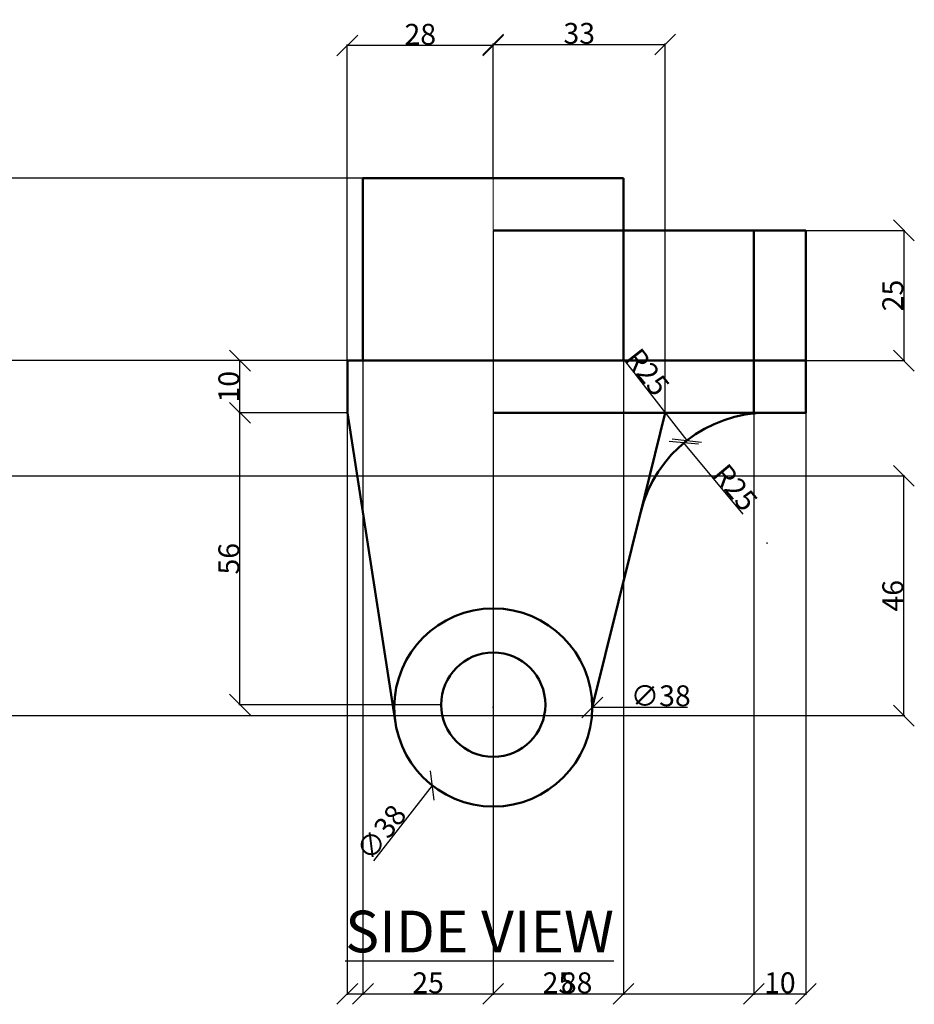
# Model space of a CAD drawing. Units: millimetres. Extents: x 113 to 503, y 39 to 409.
# Tile 3 of 3: x 332 to 503, y 39 to 228. Entities that reach past the tile are written whole.
import ezdxf

# ---------------------------------------------------------------- set-up
doc = ezdxf.new("R2010")
doc.units = ezdxf.units.MM
doc.header["$MEASUREMENT"] = 0
doc.linetypes.add('CENTER', pattern=[50.8, 31.75, -6.35, 6.35, -6.35])
for name, color, linetype, lineweight in [('M-CNTR', 1, 'CENTER', 18), ('M-DIMS', 2, 'Continuous', 25), ('M-OUTL', 7, 'Continuous', 50), ('M-TEXT', 3, 'Continuous', 25)]:
    doc.layers.add(name, color=color, linetype=linetype, lineweight=lineweight)
doc.styles.get("Standard").update_dxf_attribs({"font": 'arial.ttf'})
doc.dimstyles.get("Standard").update_dxf_attribs({"dimtxt": 4, "dimasz": 4, "dimexe": 0.18, "dimexo": 0.0625, "dimgap": 0.09, "dimtad": 1, "dimdec": 0, "dimzin": 0, "dimdsep": 46, "dimtxsty": 'Standard', "dimblk": 'OBLIQUE', "dimcen": 0.09, "dimclre": 251, "dimadec": 0, "dimazin": 0, "dimtfac": 1, "dimtdec": 0, "dimtofl": 0, "dimtmove": 0, "dimatfit": 3, "dimfxl": 1, "dimtolj": 1, "dimtzin": 0, "dimarcsym": 0})

# ---------------------------------------------------------------- blocks, each defined once
blk = doc.blocks.new('_Oblique')
at = {"color": 0, "linetype": 'ByBlock', "lineweight": -2}
blk.add_line((-0.5, -0.5), (0.5, 0.5), dxfattribs=at)
blk = doc.blocks.new('*D31')
at = {"layer": 'Defpoints', "color": 0, "transparency": 16777216}
for p in [(394.49, 223.24), (422.49, 219.68), (394.49, 162.77)]:
    blk.add_point(p, dxfattribs=at)
at = {"layer": 'M-DIMS', "color": 0, "lineweight": -2, "transparency": 16777216}
for p, q in [((394.49, 162.83), (394.49, 223.42)), ((422.49, 223.24), (394.49, 223.24)), ((422.49, 219.74), (422.49, 223.42))]:
    blk.add_line(p, q, dxfattribs=at)
at = {"layer": 'M-DIMS', "color": 0, "lineweight": -2, "transparency": 16777216, "xscale": 4, "yscale": 4, "zscale": 4, "rotation": 180}
blk.add_blockref('_Oblique', (394.49, 223.24), dxfattribs=at)
at = {"layer": 'M-DIMS', "color": 0, "lineweight": -2, "transparency": 16777216, "xscale": 4, "yscale": 4, "zscale": 4}
blk.add_blockref('_Oblique', (422.49, 223.24), dxfattribs=at)
at = {"layer": 'M-DIMS', "color": 0, "transparency": 16777216, "insert": (408.49, 225.38), "char_height": 4, "attachment_point": 5}
blk.add_mtext('\\A1;28', dxfattribs=at)
blk = doc.blocks.new('*D32')
at = {"layer": 'Defpoints', "color": 0, "transparency": 16777216}
for p in [(455.49, 223.42), (422.49, 197.77), (455.49, 152.77)]:
    blk.add_point(p, dxfattribs=at)
at = {"layer": 'M-DIMS', "color": 0, "lineweight": -2, "transparency": 16777216}
for p, q in [((422.49, 197.83), (422.49, 223.6)), ((422.49, 223.42), (455.49, 223.42)), ((455.49, 152.83), (455.49, 223.6))]:
    blk.add_line(p, q, dxfattribs=at)
at = {"layer": 'M-DIMS', "color": 0, "lineweight": -2, "transparency": 16777216, "xscale": 4, "yscale": 4, "zscale": 4, "rotation": 180}
blk.add_blockref('_Oblique', (422.49, 223.42), dxfattribs=at)
at = {"layer": 'M-DIMS', "color": 0, "lineweight": -2, "transparency": 16777216, "xscale": 4, "yscale": 4, "zscale": 4}
blk.add_blockref('_Oblique', (455.49, 223.42), dxfattribs=at)
at = {"layer": 'M-DIMS', "color": 0, "transparency": 16777216, "insert": (438.99, 225.56), "char_height": 4, "attachment_point": 5}
blk.add_mtext('\\A1;33', dxfattribs=at)
blk = doc.blocks.new('*D33')
at = {"layer": 'Defpoints', "color": 0, "transparency": 16777216}
for p in [(459.08, 147), (475.06, 127.77)]:
    blk.add_point(p, dxfattribs=at)
at = {"layer": 'M-DIMS', "color": 0, "lineweight": -2, "transparency": 16777216}
blk.add_line((470.44, 133.33), (459.08, 147), dxfattribs=at)
at = {"layer": 'M-DIMS', "color": 0, "lineweight": -2, "transparency": 16777216, "xscale": 4, "yscale": 4, "zscale": 4, "rotation": 129.7281850438319}
blk.add_blockref('_Oblique', (459.08, 147), dxfattribs=at)
at = {"layer": 'M-DIMS', "color": 0, "transparency": 16777216, "insert": (468.95, 138.45), "char_height": 4, "attachment_point": 5, "rotation": 309.7282}
blk.add_mtext('\\A1;R25', dxfattribs=at)
blk = doc.blocks.new('*D34')
at = {"layer": 'Defpoints', "color": 0, "transparency": 16777216}
for p in [(434.17, 111.23), (410.82, 81.25)]:
    blk.add_point(p, dxfattribs=at)
at = {"layer": 'M-DIMS', "color": 0, "lineweight": -2, "transparency": 16777216}
for p, q in [((422.4, 96.24), (422.58, 96.24)), ((422.49, 96.15), (422.49, 96.33)), ((399.6, 66.83), (410.82, 81.25))]:
    blk.add_line(p, q, dxfattribs=at)
at = {"layer": 'M-DIMS', "color": 0, "lineweight": -2, "transparency": 16777216, "xscale": 4, "yscale": 4, "zscale": 4, "rotation": 52.09101738177235}
blk.add_blockref('_Oblique', (410.82, 81.25), dxfattribs=at)
at = {"layer": 'M-DIMS', "color": 0, "transparency": 16777216, "insert": (400.98, 72.26), "char_height": 4, "attachment_point": 5, "rotation": 52.091}
blk.add_mtext('\\A1;∅38', dxfattribs=at)
blk = doc.blocks.new('*D35')
at = {"layer": 'Defpoints', "color": 0, "transparency": 16777216}
for p in [(373.88, 152.77), (394.49, 152.77), (412.49, 96.77)]:
    blk.add_point(p, dxfattribs=at)
at = {"layer": 'M-DIMS', "color": 0, "lineweight": -2, "transparency": 16777216}
for p, q in [((394.43, 152.77), (373.7, 152.77)), ((373.88, 96.77), (373.88, 152.77)), ((412.43, 96.77), (373.7, 96.77))]:
    blk.add_line(p, q, dxfattribs=at)
at = {"layer": 'M-DIMS', "color": 0, "lineweight": -2, "transparency": 16777216, "xscale": 4, "yscale": 4, "zscale": 4}
for p, rotation in [((373.88, 152.77), 90), ((373.88, 96.77), 270)]:
    blk.add_blockref('_Oblique', p, dxfattribs=dict(at, rotation=rotation))
at = {"layer": 'M-DIMS', "color": 0, "transparency": 16777216, "insert": (371.75, 124.77), "char_height": 4, "attachment_point": 5, "rotation": 90}
blk.add_mtext('\\A1;56', dxfattribs=at)
blk = doc.blocks.new('*D36')
at = {"layer": 'Defpoints', "color": 0, "transparency": 16777216}
for p in [(373.88, 162.77), (394.49, 162.77), (394.49, 152.77)]:
    blk.add_point(p, dxfattribs=at)
at = {"layer": 'M-DIMS', "color": 0, "lineweight": -2, "transparency": 16777216}
for p, q in [((394.43, 162.77), (373.7, 162.77)), ((373.88, 152.77), (373.88, 162.77)), ((394.43, 152.77), (373.7, 152.77))]:
    blk.add_line(p, q, dxfattribs=at)
at = {"layer": 'M-DIMS', "color": 0, "lineweight": -2, "transparency": 16777216, "xscale": 4, "yscale": 4, "zscale": 4}
for p, rotation in [((373.88, 162.77), 90), ((373.88, 152.77), 270)]:
    blk.add_blockref('_Oblique', p, dxfattribs=dict(at, rotation=rotation))
at = {"layer": 'M-DIMS', "color": 0, "transparency": 16777216, "insert": (371.75, 157.77), "char_height": 4, "attachment_point": 5, "rotation": 90}
blk.add_mtext('\\A1;10', dxfattribs=at)
blk = doc.blocks.new('*D38')
at = {"layer": 'Defpoints', "color": 0, "transparency": 16777216}
for p in [(293.81, 140.67), (501.29, 140.67), (267.81, 94.67)]:
    blk.add_point(p, dxfattribs=at)
at = {"layer": 'M-DIMS', "color": 251, "lineweight": -2, "transparency": 16777216}
for p, q in [((293.87, 140.67), (501.47, 140.67)), ((267.87, 94.67), (501.47, 94.67))]:
    blk.add_line(p, q, dxfattribs=at)
at = {"layer": 'M-DIMS', "color": 0, "lineweight": -2, "transparency": 16777216}
blk.add_line((501.29, 94.67), (501.29, 140.67), dxfattribs=at)
at = {"layer": 'M-DIMS', "color": 0, "lineweight": -2, "transparency": 16777216, "xscale": 4, "yscale": 4, "zscale": 4}
for p, rotation in [((501.29, 140.67), 90), ((501.29, 94.67), 270)]:
    blk.add_blockref('_Oblique', p, dxfattribs=dict(at, rotation=rotation))
at = {"layer": 'M-DIMS', "color": 0, "transparency": 16777216, "insert": (499.16, 117.67), "char_height": 4, "attachment_point": 5, "rotation": 90}
blk.add_mtext('\\A1;46', dxfattribs=at)
blk = doc.blocks.new('*D43')
at = {"layer": 'Defpoints', "color": 0, "transparency": 16777216}
for p in [(394.49, 162.77), (482.49, 162.77), (482.49, 41.29)]:
    blk.add_point(p, dxfattribs=at)
at = {"layer": 'M-DIMS', "color": 251, "lineweight": -2, "transparency": 16777216}
for p, q in [((394.49, 162.71), (394.49, 41.11)), ((482.49, 162.71), (482.49, 41.11))]:
    blk.add_line(p, q, dxfattribs=at)
at = {"layer": 'M-DIMS', "color": 0, "lineweight": -2, "transparency": 16777216}
blk.add_line((394.49, 41.29), (482.49, 41.29), dxfattribs=at)
at = {"layer": 'M-DIMS', "color": 0, "lineweight": -2, "transparency": 16777216, "xscale": 4, "yscale": 4, "zscale": 4, "rotation": 180}
blk.add_blockref('_Oblique', (394.49, 41.29), dxfattribs=at)
at = {"layer": 'M-DIMS', "color": 0, "lineweight": -2, "transparency": 16777216, "xscale": 4, "yscale": 4, "zscale": 4}
blk.add_blockref('_Oblique', (482.49, 41.29), dxfattribs=at)
at = {"layer": 'M-DIMS', "color": 0, "transparency": 16777216, "insert": (438.49, 43.42), "char_height": 4, "attachment_point": 5}
blk.add_mtext('\\A1;88', dxfattribs=at)
blk = doc.blocks.new('*D44')
at = {"layer": 'Defpoints', "color": 0, "transparency": 16777216}
for p in [(397.49, 197.77), (422.49, 187.77), (422.49, 41.29)]:
    blk.add_point(p, dxfattribs=at)
at = {"layer": 'M-DIMS', "color": 251, "lineweight": -2, "transparency": 16777216}
for p, q in [((397.49, 197.71), (397.49, 41.11)), ((422.49, 187.71), (422.49, 41.11))]:
    blk.add_line(p, q, dxfattribs=at)
at = {"layer": 'M-DIMS', "color": 0, "lineweight": -2, "transparency": 16777216}
blk.add_line((397.49, 41.29), (422.49, 41.29), dxfattribs=at)
at = {"layer": 'M-DIMS', "color": 0, "lineweight": -2, "transparency": 16777216, "xscale": 4, "yscale": 4, "zscale": 4, "rotation": 180}
blk.add_blockref('_Oblique', (397.49, 41.29), dxfattribs=at)
at = {"layer": 'M-DIMS', "color": 0, "lineweight": -2, "transparency": 16777216, "xscale": 4, "yscale": 4, "zscale": 4}
blk.add_blockref('_Oblique', (422.49, 41.29), dxfattribs=at)
at = {"layer": 'M-DIMS', "color": 0, "transparency": 16777216, "insert": (409.99, 43.42), "char_height": 4, "attachment_point": 5}
blk.add_mtext('\\A1;25', dxfattribs=at)
blk = doc.blocks.new('*D45')
at = {"layer": 'Defpoints', "color": 0, "transparency": 16777216}
for p in [(447.49, 197.77), (422.49, 187.77), (447.49, 41.29)]:
    blk.add_point(p, dxfattribs=at)
at = {"layer": 'M-DIMS', "color": 251, "lineweight": -2, "transparency": 16777216}
for p, q in [((447.49, 197.71), (447.49, 41.11)), ((422.49, 187.71), (422.49, 41.11))]:
    blk.add_line(p, q, dxfattribs=at)
at = {"layer": 'M-DIMS', "color": 0, "lineweight": -2, "transparency": 16777216}
blk.add_line((422.49, 41.29), (447.49, 41.29), dxfattribs=at)
at = {"layer": 'M-DIMS', "color": 0, "lineweight": -2, "transparency": 16777216, "xscale": 4, "yscale": 4, "zscale": 4, "rotation": 180}
blk.add_blockref('_Oblique', (422.49, 41.29), dxfattribs=at)
at = {"layer": 'M-DIMS', "color": 0, "lineweight": -2, "transparency": 16777216, "xscale": 4, "yscale": 4, "zscale": 4}
blk.add_blockref('_Oblique', (447.49, 41.29), dxfattribs=at)
at = {"layer": 'M-DIMS', "color": 0, "transparency": 16777216, "insert": (434.99, 43.42), "char_height": 4, "attachment_point": 5}
blk.add_mtext('\\A1;25', dxfattribs=at)
blk = doc.blocks.new('*D46')
at = {"layer": 'Defpoints', "color": 0, "transparency": 16777216}
for p in [(472.49, 187.77), (482.49, 187.77), (482.49, 41.29)]:
    blk.add_point(p, dxfattribs=at)
at = {"layer": 'M-DIMS', "color": 251, "lineweight": -2, "transparency": 16777216}
for p, q in [((472.49, 187.71), (472.49, 41.11)), ((482.49, 187.71), (482.49, 41.11))]:
    blk.add_line(p, q, dxfattribs=at)
at = {"layer": 'M-DIMS', "color": 0, "lineweight": -2, "transparency": 16777216}
blk.add_line((472.49, 41.29), (482.49, 41.29), dxfattribs=at)
at = {"layer": 'M-DIMS', "color": 0, "lineweight": -2, "transparency": 16777216, "xscale": 4, "yscale": 4, "zscale": 4, "rotation": 180}
blk.add_blockref('_Oblique', (472.49, 41.29), dxfattribs=at)
at = {"layer": 'M-DIMS', "color": 0, "lineweight": -2, "transparency": 16777216, "xscale": 4, "yscale": 4, "zscale": 4}
blk.add_blockref('_Oblique', (482.49, 41.29), dxfattribs=at)
at = {"layer": 'M-DIMS', "color": 0, "transparency": 16777216, "insert": (477.49, 43.42), "char_height": 4, "attachment_point": 5}
blk.add_mtext('\\A1;10', dxfattribs=at)
blk = doc.blocks.new('*D47')
at = {"layer": 'Defpoints', "color": 0, "transparency": 16777216}
for p in [(125.01, 197.77), (397.49, 197.77), (397.49, 162.77)]:
    blk.add_point(p, dxfattribs=at)
at = {"layer": 'M-DIMS', "color": 251, "lineweight": -2, "transparency": 16777216}
for p, q in [((397.43, 197.77), (124.83, 197.77)), ((397.43, 162.77), (124.83, 162.77))]:
    blk.add_line(p, q, dxfattribs=at)
at = {"layer": 'M-DIMS', "color": 0, "lineweight": -2, "transparency": 16777216}
blk.add_line((125.01, 162.77), (125.01, 197.77), dxfattribs=at)
at = {"layer": 'M-DIMS', "color": 0, "lineweight": -2, "transparency": 16777216, "xscale": 4, "yscale": 4, "zscale": 4}
for p, rotation in [((125.01, 197.77), 90), ((125.01, 162.77), 270)]:
    blk.add_blockref('_Oblique', p, dxfattribs=dict(at, rotation=rotation))
at = {"layer": 'M-DIMS', "color": 0, "transparency": 16777216, "insert": (122.88, 180.27), "char_height": 4, "attachment_point": 5, "rotation": 90}
blk.add_mtext('\\A1;35', dxfattribs=at)
blk = doc.blocks.new('*D48')
at = {"layer": 'Defpoints', "color": 0, "transparency": 16777216}
for p in [(482.49, 187.77), (482.49, 162.77), (501.29, 162.77)]:
    blk.add_point(p, dxfattribs=at)
at = {"layer": 'M-DIMS', "color": 251, "lineweight": -2, "transparency": 16777216}
for p, q in [((482.56, 187.77), (501.47, 187.77)), ((482.56, 162.77), (501.47, 162.77))]:
    blk.add_line(p, q, dxfattribs=at)
at = {"layer": 'M-DIMS', "color": 0, "lineweight": -2, "transparency": 16777216}
blk.add_line((501.29, 187.77), (501.29, 162.77), dxfattribs=at)
at = {"layer": 'M-DIMS', "color": 0, "lineweight": -2, "transparency": 16777216, "xscale": 4, "yscale": 4, "zscale": 4}
for p, rotation in [((501.29, 187.77), 90), ((501.29, 162.77), 270)]:
    blk.add_blockref('_Oblique', p, dxfattribs=dict(at, rotation=rotation))
at = {"layer": 'M-DIMS', "color": 0, "transparency": 16777216, "insert": (499.16, 175.27), "char_height": 4, "attachment_point": 5, "rotation": 90}
blk.add_mtext('\\A1;25', dxfattribs=at)
blk = doc.blocks.new('*D55')
at = {"layer": 'Defpoints', "color": 0, "transparency": 16777216}
for p in [(403.49, 96.24), (441.49, 96.24)]:
    blk.add_point(p, dxfattribs=at)
at = {"layer": 'M-DIMS', "color": 251, "lineweight": -2, "transparency": 16777216}
for p, q in [((422.4, 96.24), (422.58, 96.24)), ((422.49, 96.15), (422.49, 96.33))]:
    blk.add_line(p, q, dxfattribs=at)
at = {"layer": 'M-DIMS', "color": 0, "lineweight": -2, "transparency": 16777216}
blk.add_line((459.76, 96.24), (441.49, 96.24), dxfattribs=at)
at = {"layer": 'M-DIMS', "color": 0, "lineweight": -2, "transparency": 16777216, "xscale": 4, "yscale": 4, "zscale": 4, "rotation": 180.0006242224398}
blk.add_blockref('_Oblique', (441.49, 96.24), dxfattribs=at)
at = {"layer": 'M-DIMS', "color": 0, "transparency": 16777216, "insert": (454.63, 98.48), "char_height": 4, "attachment_point": 5, "rotation": 0.0006}
blk.add_mtext('\\A1;∅38', dxfattribs=at)
blk = doc.blocks.new('*D56')
at = {"layer": 'Defpoints', "color": 0, "transparency": 16777216}
for p in [(459.65, 147.46), (475.06, 127.77)]:
    blk.add_point(p, dxfattribs=at)
at = {"layer": 'M-DIMS', "color": 0, "lineweight": -2, "transparency": 16777216}
blk.add_line((447.4, 163.12), (459.65, 147.46), dxfattribs=at)
at = {"layer": 'M-DIMS', "color": 251, "lineweight": -2, "transparency": 16777216}
for p, q in [((474.97, 127.77), (475.15, 127.77)), ((475.06, 127.68), (475.06, 127.86))]:
    blk.add_line(p, q, dxfattribs=at)
at = {"layer": 'M-DIMS', "color": 0, "lineweight": -2, "transparency": 16777216, "xscale": 4, "yscale": 4, "zscale": 4, "rotation": 308.0454988541384}
blk.add_blockref('_Oblique', (459.65, 147.46), dxfattribs=at)
at = {"layer": 'M-DIMS', "color": 0, "transparency": 16777216, "insert": (452.09, 160.59), "char_height": 4, "attachment_point": 5, "rotation": 308.0455}
blk.add_mtext('\\A1;R25', dxfattribs=at)

msp = doc.modelspace()

# ---------------------------------------------------------------- linework, layer by layer
at = {"layer": 'M-CNTR'}
msp.add_line((422.495, 219.682), (422.495, 60.092), dxfattribs=at)
at = {"layer": 'M-OUTL'}
for p, q in [((397.495, 197.771), (397.495, 162.771)), ((397.495, 197.771), (447.495, 197.771)), ((447.495, 197.771), (447.495, 162.771)), ((422.495, 187.771), (482.495, 187.771)), ((472.495, 187.771), (472.495, 152.771)), ((482.495, 187.771), (482.495, 152.771)), ((394.495, 162.771), (394.495, 152.771)), ((394.495, 162.771), (482.495, 162.771)), ((394.495, 152.771), (403.719, 93.322)), ((422.495, 152.771), (482.495, 152.771)), ((451.558, 136.872), (455.495, 152.771)), ((441.495, 96.236), (451.558, 136.872))]:
    msp.add_line(p, q, dxfattribs=at)
for centre, radius in [((422.495, 96.236), 19), ((422.495, 96.771), 10)]:
    msp.add_circle(centre, radius, dxfattribs=at)
msp.add_arc((475.059, 127.771), 25, 90, 166.09153, dxfattribs=at)

# ---------------------------------------------------------------- texts
at = {"layer": 'M-TEXT', "ltscale": 5, "insert": (394.085, 57.257), "char_height": 8, "attachment_point": 1}
msp.add_mtext_dynamic_manual_height_columns('{\\LSIDE VIEW}', width=109.02237, gutter_width=1, heights=[0], dxfattribs=at)

# ---------------------------------------------------------------- dimensions: what is measured, and where the dimension line sits
at = {"layer": 'M-DIMS'}
for base, p1, p2, override, picture, middle in [((394.495, 223.245), (422.495, 219.682), (394.495, 162.771), {"dimclrd": 0, "dimclre": 0, "dimclrt": 0}, '*D31', (408.495, 225.377)), ((455.495, 223.425), (422.495, 197.771), (455.495, 152.771), {"dimclrd": 0, "dimclre": 0, "dimclrt": 0}, '*D32', (438.995, 225.558)), ((422.495, 41.292), (397.495, 197.771), (422.495, 187.771), {"dimdec": 0, "dimlfac": 1, "dimrnd": 0, "dimzin": 0, "dimdsep": 46, "dimlunit": 2}, '*D44', (409.995, 43.425)), ((447.495, 41.292), (422.495, 187.771), (447.495, 197.771), {"dimdec": 0, "dimlfac": 1, "dimrnd": 0, "dimzin": 0, "dimdsep": 46, "dimlunit": 2}, '*D45', (434.995, 43.425)), ((482.495, 41.292), (472.495, 187.771), (482.495, 187.771), {"dimdec": 0, "dimlfac": 1, "dimrnd": 0, "dimzin": 0, "dimdsep": 46, "dimlunit": 2}, '*D46', (477.495, 43.425)), ((482.495, 41.292), (394.495, 162.771), (482.495, 162.771), {"dimdec": 0, "dimlfac": 1, "dimrnd": 0, "dimzin": 0, "dimdsep": 46, "dimlunit": 2}, '*D43', (438.495, 43.425))]:
    dim = msp.add_linear_dim(base=base, p1=p1, p2=p2, dimstyle='Standard', override=override, dxfattribs=at)
    dim.commit()
    dim.dimension.update_dxf_attribs({"geometry": picture, "text_midpoint": middle})
for base, p1, p2, override, picture, middle in [((125.01, 197.771), (397.495, 162.771), (397.495, 197.771), {"dimdec": 0, "dimlfac": 1, "dimrnd": 0, "dimzin": 0, "dimdsep": 46, "dimlunit": 2}, '*D47', (122.877, 180.271)), ((501.295, 162.771), (482.495, 187.771), (482.495, 162.771), {"dimdec": 0, "dimlfac": 1, "dimrnd": 0, "dimzin": 0, "dimdsep": 46, "dimlunit": 2}, '*D48', (499.162, 175.271)), ((373.884, 162.771), (394.495, 152.771), (394.495, 162.771), {"dimclrd": 0, "dimclre": 0, "dimclrt": 0}, '*D36', (371.751, 157.771)), ((373.884, 152.771), (412.495, 96.771), (394.495, 152.771), {"dimclrd": 0, "dimclre": 0, "dimclrt": 0}, '*D35', (371.751, 124.771)), ((501.295, 140.675), (267.81, 94.675), (293.81, 140.675), {"dimdec": 0, "dimlfac": 1, "dimrnd": 0, "dimzin": 0, "dimdsep": 46, "dimlunit": 2}, '*D38', (499.162, 117.675))]:
    dim = msp.add_linear_dim(base=base, p1=p1, p2=p2, angle=90, dimstyle='Standard', override=override, dxfattribs=at)
    dim.commit()
    dim.dimension.update_dxf_attribs({"geometry": picture, "text_midpoint": middle})
for mpoint, override, picture, middle in [((459.652, 147.459), {"dimdec": 0, "dimlfac": 1, "dimrnd": 0, "dimzin": 0, "dimdsep": 46, "dimlunit": 2}, '*D56', (450.407, 159.272)), ((459.08, 146.998), {"dimclrd": 0, "dimclre": 0, "dimclrt": 0}, '*D33', (467.315, 137.09))]:
    dim = msp.add_radius_dim(center=(475.059, 127.771), mpoint=mpoint, dimstyle='Standard', override=override, dxfattribs=at)
    dim.commit()
    dim.dimension.update_dxf_attribs({"geometry": picture, "text_midpoint": middle, "dimtype": 164})
for p1, p2, override, picture, middle in [((434.168, 111.227), (410.821, 81.245), {"dimclrd": 0, "dimclre": 0, "dimclrt": 0}, '*D34', (400.98, 72.26)), ((403.495, 96.236), (441.495, 96.236), {"dimdec": 0, "dimlfac": 1, "dimrnd": 0, "dimzin": 0, "dimdsep": 46, "dimlunit": 2}, '*D55', (454.63, 96.236))]:
    dim = msp.add_diameter_dim_2p(p1=p1, p2=p2, dimstyle='Standard', override=override, dxfattribs=at)
    dim.commit()
    dim.dimension.update_dxf_attribs({"geometry": picture, "text_midpoint": middle})

doc.saveas('drawing.dxf')
